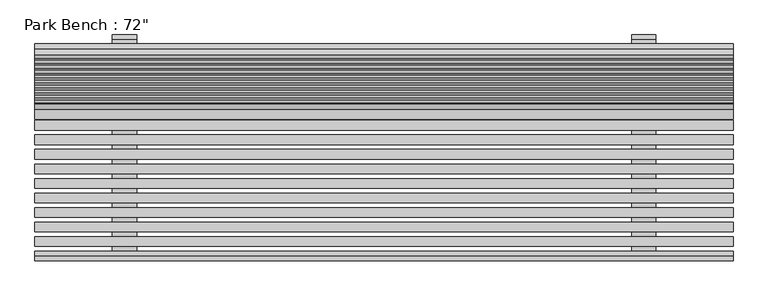
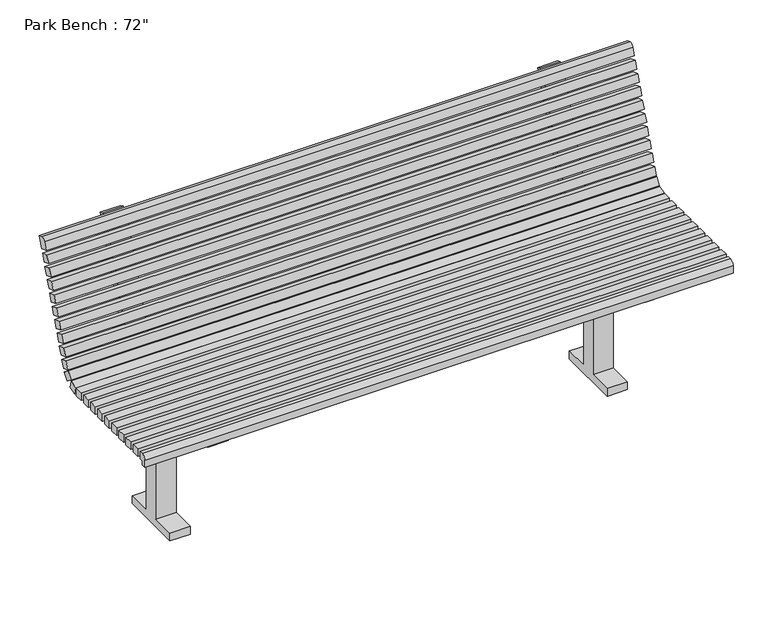
"""IFC4 building model written with IfcOpenShell, lengths in millimetres: geographic element geometry."""

from ifc_helpers import new_model, si_unit, point, frame, frame_2d, origin, place, context, project, spatial, polyline, circle_curve, trimmed, segment, composite_curve, outline, extrude, source, transform, mapped, element, save


def geographic_element_235d1464(model_context):
    return source(origin(), model_context, "Body", "SweptSolid", [
        extrude(outline(polyline([(914.4, -255.4337104), (914.4, -280.8337104), (-914.4, -280.8337104), (-914.4, -255.4337104), (914.4, -255.4337104)])), frame((0.0, 0.0, 457.2), z_axis=(0.0, 0.0, 1.0), x_axis=(1.0, 0.0, 0.0)), (0.0, 0.0, 1.0), 25.4),
        extrude(outline(polyline([(914.4, -217.3337104), (914.4, -242.7337104), (-914.4, -242.7337104), (-914.4, -217.3337104), (914.4, -217.3337104)])), frame((0.0, 0.0, 457.2), z_axis=(0.0, 0.0, 1.0), x_axis=(1.0, 0.0, 0.0)), (0.0, 0.0, 1.0), 25.4),
        extrude(outline(polyline([(914.4, -179.2337104), (914.4, -204.6337104), (-914.4, -204.6337104), (-914.4, -179.2337104), (914.4, -179.2337104)])), frame((0.0, 0.0, 457.2), z_axis=(0.0, 0.0, 1.0), x_axis=(1.0, 0.0, 0.0)), (0.0, 0.0, 1.0), 25.4),
        extrude(outline(polyline([(914.4, -141.1337104), (914.4, -166.5337104), (-914.4, -166.5337104), (-914.4, -141.1337104), (914.4, -141.1337104)])), frame((0.0, 0.0, 457.2), z_axis=(0.0, 0.0, 1.0), x_axis=(1.0, 0.0, 0.0)), (0.0, 0.0, 1.0), 25.4),
        extrude(outline(polyline([(914.4, -103.0337104), (914.4, -128.4337104), (-914.4, -128.4337104), (-914.4, -103.0337104), (914.4, -103.0337104)])), frame((0.0, 0.0, 457.2), z_axis=(0.0, 0.0, 1.0), x_axis=(1.0, 0.0, 0.0)), (0.0, 0.0, 1.0), 25.4),
        extrude(outline(polyline([(914.4, -64.9337104), (914.4, -90.3337104), (-914.4, -90.3337104), (-914.4, -64.9337104), (914.4, -64.9337104)])), frame((0.0, 0.0, 457.2), z_axis=(0.0, 0.0, 1.0), x_axis=(1.0, 0.0, 0.0)), (0.0, 0.0, 1.0), 25.4),
        extrude(outline(polyline([(914.4, -26.8337104), (914.4, -52.2337104), (-914.4, -52.2337104), (-914.4, -26.8337104), (914.4, -26.8337104)])), frame((0.0, 0.0, 457.2), z_axis=(0.0, 0.0, 1.0), x_axis=(1.0, 0.0, 0.0)), (0.0, 0.0, 1.0), 25.4),
        extrude(outline(polyline([(914.4, 11.2662896), (914.4, -14.1337104), (-914.4, -14.1337104), (-914.4, 11.2662896), (914.4, 11.2662896)])), frame((0.0, 0.0, 457.2), z_axis=(0.0, 0.0, 1.0), x_axis=(1.0, 0.0, 0.0)), (0.0, 0.0, 1.0), 25.4),
        extrude(outline(polyline([(914.4, 49.3662896), (914.4, 23.9662896), (-914.4, 23.9662896), (-914.4, 49.3662896), (914.4, 49.3662896)])), frame((0.0, 0.0, 457.2), z_axis=(0.0, 0.0, 1.0), x_axis=(1.0, 0.0, 0.0)), (0.0, 0.0, 1.0), 25.4),
        extrude(outline(composite_curve([segment(polyline([(-304.8, 457.2), (-304.8, 444.5), (-318.9337104, 444.5), (-318.9337104, 468.3125)]), True, "CONTINUOUS"), segment(trimmed(circle_curve(frame_2d((-304.6462104, 468.3125)), 14.2875), [point((-318.9337104, 468.3125))], [point((-304.6462104, 482.6))], False, "CARTESIAN"), True, "CONTINUOUS"), segment(polyline([(-304.6462104, 482.6), (-293.5337104, 482.6), (-293.5337104, 457.2), (-304.8, 457.2)]), True, "CONTINUOUS")], self_intersect=False)), frame((-914.4, 0.0, 0.0), z_axis=(1.0, 0.0, 0.0), x_axis=(0.0, 1.0, 0.0)), (0.0, 0.0, 1.0), 1828.8),
        extrude(outline(polyline([(0.0, -25.4), (0.0, 0.0), (1828.8, 0.0), (1828.8, -25.4), (0.0, -25.4)])), frame((914.4, 121.2738625, 585.5181247), z_axis=(0.0, 0.342020143325687, 0.9396926207859018), x_axis=(-1.0, 0.0, 0.0)), (0.0, 0.0, 1.0), 25.4),
        extrude(outline(polyline([(0.0, -25.4), (0.0, 0.0), (1828.8, 0.0), (1828.8, -25.4), (0.0, -25.4)])), frame((914.4, 134.30483, 621.3204136), z_axis=(0.0, 0.34202014332568254, 0.9396926207859034), x_axis=(-1.0, 0.0, 0.0)), (0.0, 0.0, 1.0), 25.4),
        extrude(outline(polyline([(0.0, -25.3999999), (0.0, 0.0), (1828.8, 0.0), (1828.8, -25.3999999), (0.0, -25.3999999)])), frame((914.4, 95.2119276, 513.913547), z_axis=(0.0, 0.34202014332568254, 0.9396926207859034), x_axis=(-1.0, 0.0, 0.0)), (0.0, 0.0, 1.0), 25.4),
        extrude(outline(polyline([(0.0, -25.4000001), (0.0, 0.0), (1828.8, 0.0), (1828.8, -25.4000001), (0.0, -25.4000001)])), frame((914.4, 108.242895, 549.7158359), z_axis=(0.0, 0.34202014332567804, 0.9396926207859051), x_axis=(-1.0, 0.0, 0.0)), (0.0, 0.0, 1.0), 25.4),
        extrude(outline(polyline([(0.0, -25.4), (0.0, 0.0), (1828.8, 0.0), (1828.8, -25.4), (0.0, -25.4)])), frame((914.4, 173.3977323, 728.7272801), z_axis=(0.0, 0.34202014332568337, 0.9396926207859031), x_axis=(-1.0, 0.0, 0.0)), (0.0, 0.0, 1.0), 25.4),
        extrude(outline(polyline([(0.0, -25.4000001), (0.0, 0.0), (1828.8, 0.0), (1828.8, -25.4000001), (0.0, -25.4000001)])), frame((914.4, 186.4286998, 764.529569), z_axis=(0.0, 0.3420201433256829, 0.9396926207859032), x_axis=(-1.0, 0.0, 0.0)), (0.0, 0.0, 1.0), 25.4),
        extrude(outline(polyline([(0.0, -25.4), (0.0, 0.0), (1828.8, 0.0), (1828.8, -25.4), (0.0, -25.4)])), frame((914.4, 147.3357974, 657.1227024), z_axis=(0.0, 0.3420201433256776, 0.9396926207859052), x_axis=(-1.0, 0.0, 0.0)), (0.0, 0.0, 1.0), 25.4),
        extrude(outline(polyline([(0.0, -25.4), (0.0, 0.0), (1828.8, 0.0), (1828.8, -25.4), (0.0, -25.4)])), frame((914.4, 160.3667649, 692.9249913), z_axis=(0.0, 0.34202014332568254, 0.9396926207859034), x_axis=(-1.0, 0.0, 0.0)), (0.0, 0.0, 1.0), 25.4),
        extrude(outline(polyline([(0.0, -25.3999999), (0.0, 0.0), (1828.8, 0.0), (1828.8, -25.3999999), (0.0, -25.3999999)])), frame((914.4, 199.4596673, 800.3318578), z_axis=(0.0, 0.3420201433256774, 0.9396926207859052), x_axis=(-1.0, 0.0, 0.0)), (0.0, 0.0, 1.0), 25.4),
        extrude(outline(composite_curve([segment(polyline([(249.3897948, 863.2491239), (236.3588273, 827.4468351), (212.4906347, 836.1341467), (221.1779464, 860.0023393)]), True, "CONTINUOUS"), segment(trimmed(circle_curve(frame_2d((233.1120426, 855.6586834)), 12.7), [point((221.1779464, 860.0023393))], [point((237.4556985, 867.5927797))], False, "CARTESIAN"), True, "CONTINUOUS"), segment(polyline([(237.4556985, 867.5927797), (249.3897948, 863.2491239)]), True, "CONTINUOUS")], self_intersect=False)), frame((-914.4, 0.0, 0.0), z_axis=(1.0, 0.0, 0.0), x_axis=(0.0, 1.0, 0.0)), (0.0, 0.0, 1.0), 1828.8),
        extrude(outline(polyline([(0.0, -25.4), (0.0, 0.0), (1828.8, 0.0), (1828.8, -25.4), (0.0, -25.4)])), frame((914.4, 78.7855779, 490.7267336), z_axis=(0.0, 0.5735764363510742, 0.8191520442889721), x_axis=(-1.0, 0.0, 0.0)), (0.0, 0.0, 1.0), 25.4),
        extrude(outline(polyline([(0.0, -25.4), (0.0, 0.0), (1828.8, 0.0), (1828.8, -25.4), (0.0, -25.4)])), frame((914.4, 59.0817015, 457.2297909), z_axis=(0.0, -0.2588190451024684, 0.9659258262890824), x_axis=(-1.0, 0.0, 0.0)), (0.0, 0.0, 1.0), 25.4),
        extrude(outline(composite_curve([segment(polyline([(-101.6, 25.4), (-25.4, 25.4), (-25.4, 431.8), (-304.8, 431.8), (-304.8, 457.2), (57.1368213, 457.2)]), True, "CONTINUOUS"), segment(trimmed(circle_curve(frame_2d((57.1368213, 520.7)), 63.5), [point((57.1368213, 457.2))], [point((116.8073027, 498.9817209))], True, "CARTESIAN"), True, "CONTINUOUS"), segment(polyline([(116.8073027, 498.9817209), (244.9406421, 851.0251774)]), True, "CONTINUOUS"), segment(trimmed(circle_curve(frame_2d((256.8747384, 846.6815216)), 12.7), [point((244.9406421, 851.0251774))], [point((261.2183942, 858.6156178))], False, "CARTESIAN"), True, "CONTINUOUS"), segment(polyline([(261.2183942, 858.6156178), (273.1524905, 854.271962), (140.6754953, 490.2944093)]), True, "CONTINUOUS"), segment(trimmed(circle_curve(frame_2d((57.1368213, 520.7)), 88.9), [point((140.6754953, 490.2944093))], [point((57.1368213, 431.8))], False, "CARTESIAN"), True, "CONTINUOUS"), segment(polyline([(57.1368213, 431.8), (25.4, 431.8), (25.4, 25.4), (101.6, 25.4), (101.6, 0.0), (-101.6, 0.0), (-101.6, 25.4)]), True, "CONTINUOUS")], self_intersect=False)), frame((648.3736591, 0.0, 0.0), z_axis=(1.0, 0.0, 0.0), x_axis=(0.0, 1.0, 0.0)), (0.0, 0.0, 1.0), 62.8263409),
        extrude(outline(composite_curve([segment(polyline([(-101.6, 25.4), (-25.4, 25.4), (-25.4, 431.8), (-304.8, 431.8), (-304.8, 457.2), (57.1368213, 457.2)]), True, "CONTINUOUS"), segment(trimmed(circle_curve(frame_2d((57.1368213, 520.7)), 63.5), [point((57.1368213, 457.2))], [point((116.8073027, 498.9817209))], True, "CARTESIAN"), True, "CONTINUOUS"), segment(polyline([(116.8073027, 498.9817209), (244.9406421, 851.0251774)]), True, "CONTINUOUS"), segment(trimmed(circle_curve(frame_2d((256.8747384, 846.6815216)), 12.7), [point((244.9406421, 851.0251774))], [point((261.2183942, 858.6156178))], False, "CARTESIAN"), True, "CONTINUOUS"), segment(polyline([(261.2183942, 858.6156178), (273.1524905, 854.271962), (140.6754953, 490.2944093)]), True, "CONTINUOUS"), segment(trimmed(circle_curve(frame_2d((57.1368213, 520.7)), 88.9), [point((140.6754953, 490.2944093))], [point((57.1368213, 431.8))], False, "CARTESIAN"), True, "CONTINUOUS"), segment(polyline([(57.1368213, 431.8), (25.4, 431.8), (25.4, 25.4), (101.6, 25.4), (101.6, 0.0), (-101.6, 0.0), (-101.6, 25.4)]), True, "CONTINUOUS")], self_intersect=False)), frame((-711.2, 0.0, 0.0), z_axis=(1.0, 0.0, 0.0), x_axis=(0.0, 1.0, 0.0)), (0.0, 0.0, 1.0), 63.8916859),
    ])


if __name__ == "__main__":
    model = new_model("IFC4")
    model_context = context("Model", 3, world=origin())
    ifc_project = project(units=[si_unit("LENGTHUNIT", "METRE", prefix="MILLI")], contexts=[model_context])
    site = spatial("IfcSite", under=ifc_project)
    building = spatial("IfcBuilding", under=site)
    placement = place(None, origin())
    geographic_element_shape = geographic_element_235d1464(model_context)
    element("IfcGeographicElement", 1, ObjectType="Park Bench : 72\"", at=placement, inside=building, context=model_context, shape_type="MappedRepresentation", body=[
        mapped(geographic_element_shape, transform((0.0, 0.0, 0.0), x_axis=(1.0, 0.0, 0.0), y_axis=(0.0, 1.0, 0.0), z_axis=(0.0, 0.0, 1.0))),
    ])
    save(model, "model.ifc")

# Revit data of these elements
# Type "Park Bench : 72\""
#   Length = 6' - 0"
#   Seat Material = Wood - Teak
#   Frame Material = Steel, Paint Finish, Dark Gray, Matte
# Element 1 (IfcGeographicElement, "Park Bench : 72\"")
#   Materials on its faces: "Wood - Teak", "Steel, Paint Finish, Dark Gray, Matte"
# Materials
#   "Wood - Teak": class "Wood", colour RGB 120 73 19, transparency 0
#   "Steel, Paint Finish, Dark Gray, Matte": class "Metal", colour RGB 0 0 0, transparency 0, Description = "Steel, paint finish, dark gray, matte", Cost = 0
